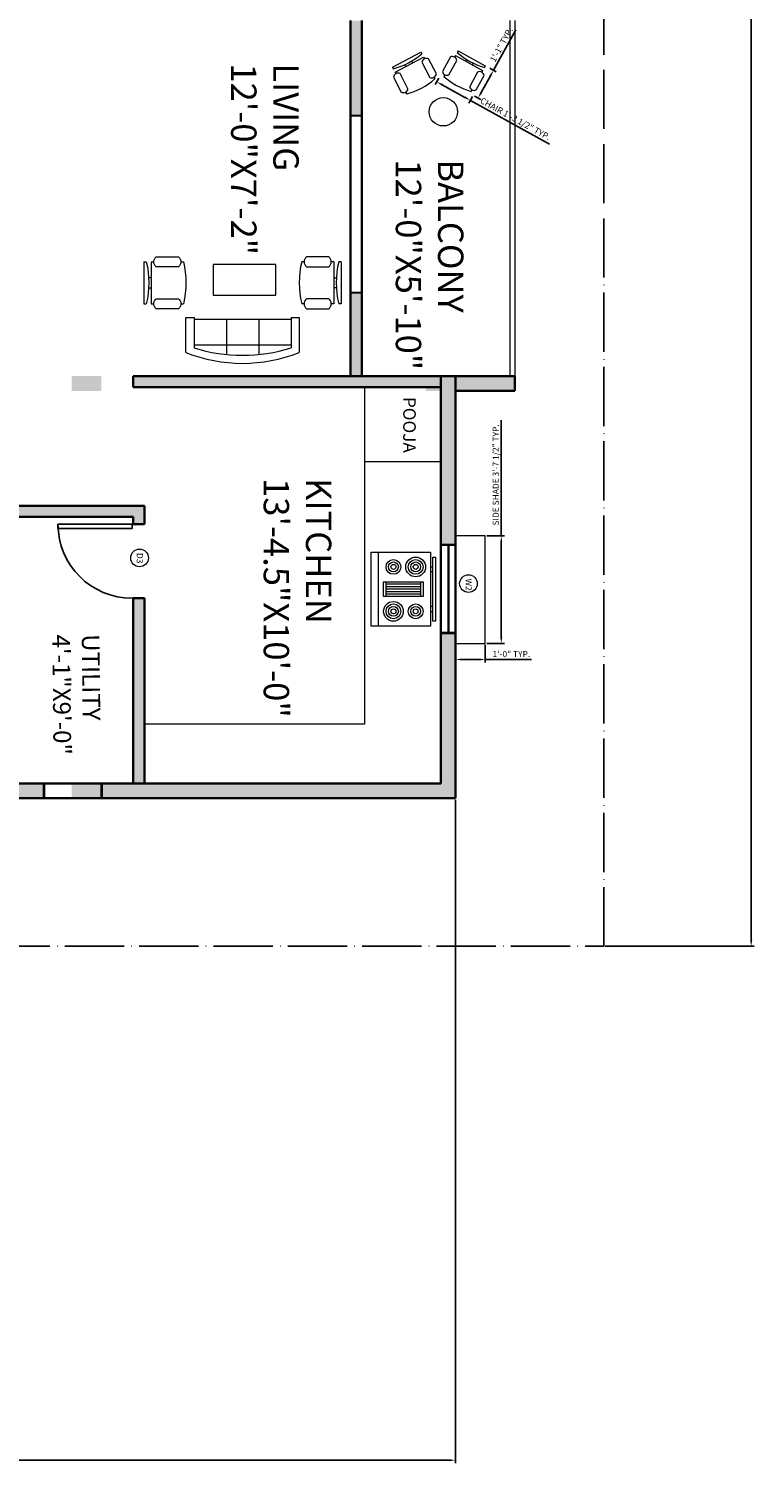
# Model space of a CAD drawing. Units: inches. Extents: x 7028582 to 7030319, y 63109697 to 63111305.
# Tile 7 of 18: x 7030003 to 7030297, y 63109697 to 63110278. Entities that reach past the tile are written whole.
import ezdxf

# ---------------------------------------------------------------- set-up
doc = ezdxf.new("R2010")
doc.units = ezdxf.units.IN
doc.linetypes.add('ACAD_ISO04W100', pattern=[30, 24, -3, 0, -3])
for name, color, linetype, lineweight in [('A-AREA-IDEN', 7, 'Continuous', 18), ('A-DOOR-IDEN', 20, 'Continuous', 13), ('A-EQPM', 9, 'Continuous', 18), ('A-FLOR-CASE', 9, 'Continuous', 18), ('A-FLOR-HRAL', 5, 'Continuous', 18), ('A-GLAZ-IDEN', 20, 'Continuous', 13), ('A-WALL-PATT', 8, 'Continuous', 13), ('C-ANNO-DIMS', 7, 'Continuous', 18), ('C-PROP', 1, 'ACAD_ISO04W100', 25), ('doors', 20, 'Continuous', 25), ('furniture', 9, 'Continuous', 18), ('S-COLS-PATT', 220, 'Continuous', 100), ('walls', 6, 'Continuous', 35), ('WINDOW SHADOW', 9, 'Continuous', 13), ('windows', 5, 'Continuous', 18)]:
    doc.layers.add(name, color=color, linetype=linetype, lineweight=lineweight)
doc.styles.get("Standard").update_dxf_attribs({"font": 'arial.ttf'})
doc.dimstyles.new('ISO-25', dxfattribs={"dimtxt": 2.5, "dimasz": 2.5, "dimexe": 1.25, "dimexo": 0.625, "dimtad": 1, "dimlunit": 4, "dimtxsty": 'Standard', "dimcen": 2.5, "dimadec": 0, "dimazin": 0, "dimtfac": 1, "dimtmove": 0, "dimatfit": 3, "dimfxl": 1, "dimarcsym": 0})

# ---------------------------------------------------------------- blocks, each defined once
blk = doc.blocks.new('*U2')
for p, q in [((0, 0), (0, -5)), ((30, 0), (30, -5))]:
    blk.add_line(p, q)
blk.add_lwpolyline([(0, 0), (0, 30), (1.75, 30), (1.75, 0)], close=True)
blk.add_arc((0, 0), 30, 0, 90)
blk = doc.blocks.new('Range-Oven - 30 in top')
for p, q in [((0, -3), (30, -3)), ((12, -6), (18, -6)), ((13, -20), (13, -6)), ((14, -6), (14, -20)), ((15, -20), (15, -6)), ((16, -6), (16, -20)), ((17, -20), (17, -6)), ((18, -20), (12, -20)), ((6, -24), (6, -25)), ((8, -25), (8, -24)), ((22, -25), (22, -24)), ((24, -24), (24, -25))]:
    blk.add_line(p, q)
for points in [[(0, -24), (0, 0), (30, 0), (30, -24)], [(12, -21), (12, -5), (18, -5), (18, -21)], [(2, -26), (2, -25), (28, -25), (28, -26)]]:
    blk.add_lwpolyline(points, close=True)
for centre, radius in [((6, -9), 4), ((6, -9), 3), ((6, -9), 2), ((6, -9), 1), ((24, -9), 3), ((24, -9), 2), ((24, -9), 1), ((6, -18), 3), ((6, -18), 2), ((6, -18), 1), ((24, -18), 4), ((24, -18), 3), ((24, -18), 2), ((24, -18), 1)]:
    blk.add_circle(centre, radius)
blk = doc.blocks.new('Chair - Desk')
for p, q in [((-8.5, 0), (-8.5, -1)), ((-8.5, 0), (8.5, 0)), ((8.5, 0), (8.5, -1)), ((-10.5, -5), (-10.5, -14)), ((-8.5, -3), (-8.5, -4)), ((-8.5, -3), (8.5, -3)), ((-6.5, -14), (-6.5, -5)), ((-2, -3), (-2, -1.9355)), ((2, -1.9576), (2, -3)), ((6.5, -5), (6.5, -14)), ((8.5, -3), (8.5, -4)), ((10.5, -14), (10.5, -5)), ((-8.5, -15), (-8.5, -16)), ((8.5, -15), (8.5, -16))]:
    blk.add_line(p, q)
for centre, radius, start, end in [((-8.5, -6.5), 2.5, 36.8699, 143.1301), ((0, 34.625), 36.625, 256.5803, 283.4197), ((8.5, -6.5), 2.5, 36.8699, 143.1301), ((-8.5, -12.5), 2.5, 216.8699, 323.1301), ((0, 19.625), 36.625, 256.5803, 283.4197), ((8.5, -12.5), 2.5, 216.8699, 323.1301)]:
    blk.add_arc(centre, radius, start, end)
blk = doc.blocks.new('Sofa - Roundback 7 ft.')
for p, q in [((-12.00002, -32.4421), (-12.00003, -6.5971)), ((11.99997, -32.4421), (11.99998, -6.5971)), ((-36.000027, -34), (-36.000027, -11.4696)), ((-35.999844, -13.3819), (35.9998, -13.3819)), ((35.99998, -34), (35.99998, -11.4696)), ((-36.000027, -32.4421), (35.99998, -32.4421))]:
    blk.add_line(p, q)
for points in [[(-36.000027, -34), (-42.000027, -34), (-42.000027, -8)], [(41.99998, -8), (41.99998, -34), (35.99998, -34)]]:
    blk.add_lwpolyline(points)
for centre, radius, start, end in [((0, -114.25), 114.25, 68.43141, 111.5686), ((-0.00001, -127.1968), 121.1968, 72.72033, 107.2797)]:
    blk.add_arc(centre, radius, start, end)
blk = doc.blocks.new('*D10')
at = {"layer": 'C-ANNO-DIMS', "color": 0, "lineweight": -2, "transparency": 16777216}
for p, q in [((7030236.33, 63111093.06), (7030296.71, 63111093.06)), ((7030295.46, 63111090.56), (7030295.46, 63109909.06)), ((7030236.33, 63109906.56), (7030296.71, 63109906.56))]:
    blk.add_line(p, q, dxfattribs=at)
at = {"layer": 'C-ANNO-DIMS', "color": 0, "lineweight": 100, "transparency": 16777216}
for points in [[(7030295.04, 63111090.56), (7030295.88, 63111090.56), (7030295.46, 63111093.06)], [(7030295.04, 63109909.06), (7030295.88, 63109909.06), (7030295.46, 63109906.56)]]:
    blk.add_solid(points, dxfattribs=at)
at = {"layer": 'Defpoints', "color": 0, "lineweight": 100, "transparency": 16777216}
for p in [(7030235.71, 63111093.06), (7030235.71, 63109906.56), (7030295.46, 63109906.56)]:
    blk.add_point(p, dxfattribs=at)
at = {"layer": 'C-ANNO-DIMS', "color": 0, "transparency": 16777216, "insert": (7030280.69, 63110499.81), "char_height": 12, "attachment_point": 5, "rotation": 90}
blk.add_mtext('98\'-10{\\H1x;\\S1/2;}"', dxfattribs=at)
blk = doc.blocks.new('WIN-SASH-36')
for p, q in [((0, 36.05), (0, 0)), ((6, 35.55), (0, 35.55)), ((2.8, 35.55), (2.8, 0.5)), ((3.2, 35.55), (3.2, 0.5)), ((6, 0), (6, 36.05)), ((0, 0.5), (6, 0.5))]:
    blk.add_line(p, q)
blk = doc.blocks.new('WIN-SASH-24-FRAME')
for p, q in [((24.05, 6), (0, 6)), ((0.5, 6), (0.5, 0)), ((23.55, 0), (23.55, 6)), ((0, 0), (24.05, 0))]:
    blk.add_line(p, q)
blk = doc.blocks.new('WIN-SASH-BALCONY')
for p, q in [((0.13, 72.09), (0.13, 36.05)), ((4.63, 71.71), (0.13, 71.71)), ((4.63, 36.05), (4.63, 72.09)), ((0, 0.02), (0.13, 36.05)), ((0.13, 35.68), (0.13, 35.68)), ((4.63, 36.04), (4.5, 0)), ((4.5, 0.37), (0, 0.39))]:
    blk.add_line(p, q)
blk = doc.blocks.new('WINDOW-SHADE-SIDE-44')
for p, q in [((12, 43.55), (0, 43.55)), ((12, 0), (12, 43.55)), ((0, 0), (12, 0))]:
    blk.add_line(p, q)
blk = doc.blocks.new('KITCHEN-COUNTER')
for p, q in [((89.09, 136.54), (89.09, 16.65)), ((120, 106.35), (89.09, 106.35)), ((89.09, 16.65), (89.09, 0)), ((89.09, 0), (0, 0))]:
    blk.add_line(p, q)
blk = doc.blocks.new('BALCONY-GUARD-12FT')
for p, q in [((0, 144), (0, 0)), ((2, 144), (2, 0))]:
    blk.add_line(p, q)
blk = doc.blocks.new('TABLE-COFFEE-RECT')
blk.add_lwpolyline([(25.34, 12.34), (0, 12.34), (0, 0), (25.34, 0)], close=True)
blk = doc.blocks.new('TAG-D3-MT-R')
blk.add_circle((3.58, 3.58), 3.58)
at = {"insert": (4.93, 5.6), "char_height": 2.5, "attachment_point": 1, "rotation": 270}
blk.add_mtext_dynamic_manual_height_columns('D3', width=2.5021, gutter_width=12.5, heights=[0], dxfattribs=at)
blk = doc.blocks.new('TAG-W2-MT-R')
blk.add_circle((3.58, 3.58), 3.58)
at = {"insert": (4.93, 5.6), "char_height": 2.5, "attachment_point": 1, "rotation": 270}
blk.add_mtext_dynamic_manual_height_columns('W2', width=2.5021, gutter_width=12.5, heights=[0], dxfattribs=at)
blk = doc.blocks.new('TABLE-BALCONY-ROUND')
blk.add_circle((5.75, 5.75), 5.75)
blk = doc.blocks.new('*D51')
at = {"layer": 'C-ANNO-DIMS', "color": 0, "lineweight": -2, "transparency": 16777216}
for p, q in [((7030168.91, 63110258.28), (7030167.48, 63110255.69)), ((7030170.28, 63110255.57), (7030179.52, 63110250.47)), ((7030182.54, 63110250.76), (7030181.11, 63110248.17)), ((7030181.71, 63110249.26), (7030213.77, 63110231.56))]:
    blk.add_line(p, q, dxfattribs=at)
at = {"layer": 'C-ANNO-DIMS', "color": 0, "lineweight": 100, "transparency": 16777216}
for points in [[(7030170.48, 63110255.94), (7030170.08, 63110255.21), (7030168.09, 63110256.78)], [(7030179.72, 63110250.84), (7030179.32, 63110250.11), (7030181.71, 63110249.26)]]:
    blk.add_solid(points, dxfattribs=at)
at = {"layer": 'Defpoints', "color": 0, "lineweight": 100, "transparency": 16777216}
for p in [(7030169.22, 63110258.83), (7030181.71, 63110249.26), (7030182.84, 63110251.31)]:
    blk.add_point(p, dxfattribs=at)
at = {"layer": 'C-ANNO-DIMS', "color": 0, "transparency": 16777216, "insert": (7030199.76, 63110241.49), "char_height": 2.5, "attachment_point": 5, "rotation": 331.10029}
blk.add_mtext('CHAIR 1\'-3 1/2" TYP.', dxfattribs=at)
blk = doc.blocks.new('*D52')
at = {"layer": 'C-ANNO-DIMS', "color": 0, "lineweight": -2, "transparency": 16777216}
for p, q in [((7030191.09, 63110261.42), (7030200.15, 63110277.84)), ((7030186.09, 63110252.37), (7030189.88, 63110259.23)), ((7030189.59, 63110262.25), (7030192.18, 63110260.82)), ((7030183.39, 63110251), (7030185.98, 63110249.57))]:
    blk.add_line(p, q, dxfattribs=at)
at = {"layer": 'C-ANNO-DIMS', "color": 0, "lineweight": 100, "transparency": 16777216}
for points in [[(7030189.52, 63110259.43), (7030190.24, 63110259.03), (7030191.09, 63110261.42)], [(7030185.72, 63110252.57), (7030186.45, 63110252.17), (7030184.88, 63110250.18)]]:
    blk.add_solid(points, dxfattribs=at)
at = {"layer": 'Defpoints', "color": 0, "lineweight": 100, "transparency": 16777216}
for p in [(7030189.04, 63110262.55), (7030191.09, 63110261.42), (7030182.84, 63110251.31)]:
    blk.add_point(p, dxfattribs=at)
at = {"layer": 'C-ANNO-DIMS', "color": 0, "transparency": 16777216, "insert": (7030194.58, 63110271.63), "char_height": 2.5, "attachment_point": 5, "rotation": 61.10029}
blk.add_mtext('1\'-1" TYP.', dxfattribs=at)
blk = doc.blocks.new('*D71')
at = {"layer": 'C-ANNO-DIMS', "color": 0, "lineweight": -2, "transparency": 16777216}
for p, q in [((7030194.24, 63110072.83), (7030194.24, 63110119.76)), ((7030188.33, 63110072.83), (7030195.49, 63110072.83)), ((7030194.24, 63110031.78), (7030194.24, 63110070.33)), ((7030188.33, 63110029.28), (7030195.49, 63110029.28))]:
    blk.add_line(p, q, dxfattribs=at)
at = {"layer": 'C-ANNO-DIMS', "color": 0, "lineweight": 100, "transparency": 16777216}
for points in [[(7030193.82, 63110070.33), (7030194.65, 63110070.33), (7030194.24, 63110072.83)], [(7030193.82, 63110031.78), (7030194.65, 63110031.78), (7030194.24, 63110029.28)]]:
    blk.add_solid(points, dxfattribs=at)
at = {"layer": 'Defpoints', "color": 0, "lineweight": 100, "transparency": 16777216}
for p in [(7030187.71, 63110072.83), (7030194.24, 63110072.83), (7030187.71, 63110029.28)]:
    blk.add_point(p, dxfattribs=at)
at = {"layer": 'C-ANNO-DIMS', "color": 0, "transparency": 16777216, "insert": (7030192.32, 63110097.54), "char_height": 2.5, "attachment_point": 5, "rotation": 90}
blk.add_mtext('SIDE SHADE 3\'-7 1/2" TYP.', dxfattribs=at)
blk = doc.blocks.new('*D72')
at = {"layer": 'C-ANNO-DIMS', "color": 0, "lineweight": -2, "transparency": 16777216}
for p, q in [((7030175.71, 63110028.66), (7030175.71, 63110021.5)), ((7030187.71, 63110028.66), (7030187.71, 63110021.5)), ((7030178.21, 63110022.75), (7030185.21, 63110022.75)), ((7030187.71, 63110022.75), (7030206.46, 63110022.75))]:
    blk.add_line(p, q, dxfattribs=at)
at = {"layer": 'C-ANNO-DIMS', "color": 0, "lineweight": 100, "transparency": 16777216}
for points in [[(7030178.21, 63110023.16), (7030178.21, 63110022.33), (7030175.71, 63110022.75)], [(7030185.21, 63110023.16), (7030185.21, 63110022.33), (7030187.71, 63110022.75)]]:
    blk.add_solid(points, dxfattribs=at)
at = {"layer": 'Defpoints', "color": 0, "lineweight": 100, "transparency": 16777216}
for p in [(7030175.71, 63110029.28), (7030187.71, 63110029.28), (7030187.71, 63110022.75)]:
    blk.add_point(p, dxfattribs=at)
at = {"layer": 'C-ANNO-DIMS', "color": 0, "transparency": 16777216, "insert": (7030198.33, 63110024.65), "char_height": 2.5, "attachment_point": 5}
blk.add_mtext('1\'-0" TYP.', dxfattribs=at)
blk = doc.blocks.new('*D99')
at = {"layer": 'C-ANNO-DIMS', "color": 0, "lineweight": -2, "transparency": 16777216}
for p, q in [((7029234.71, 63109965.93), (7029234.71, 63109697.14)), ((7030175.71, 63109965.93), (7030175.71, 63109697.14)), ((7029237.21, 63109698.39), (7030173.21, 63109698.39))]:
    blk.add_line(p, q, dxfattribs=at)
at = {"layer": 'C-ANNO-DIMS', "color": 0, "lineweight": 100, "transparency": 16777216}
for points in [[(7029237.21, 63109698.8), (7029237.21, 63109697.97), (7029234.71, 63109698.39)], [(7030173.21, 63109698.8), (7030173.21, 63109697.97), (7030175.71, 63109698.39)]]:
    blk.add_solid(points, dxfattribs=at)
at = {"layer": 'Defpoints', "color": 0, "lineweight": 100, "transparency": 16777216}
for p in [(7029234.71, 63109966.56), (7030175.71, 63109966.56), (7030175.71, 63109698.39)]:
    blk.add_point(p, dxfattribs=at)
at = {"layer": 'C-ANNO-DIMS', "color": 0, "transparency": 16777216, "insert": (7029705.21, 63109700.29), "char_height": 2.5, "attachment_point": 5}
blk.add_mtext('78\'-5"', dxfattribs=at)

msp = doc.modelspace()

# ---------------------------------------------------------------- hatches: boundary and pattern name
at = {"layer": 'A-WALL-PATT'}
h = msp.add_hatch(color=256, dxfattribs=at)
h.dxf.hatch_style = 1
h.paths.add_polyline_path([(7030137.705, 63110281.557), (7030133.205, 63110281.557), (7030133.205, 63110243.163), (7030137.705, 63110243.163)])
h = msp.add_hatch(color=256, dxfattribs=at)
h.dxf.hatch_style = 1
h.paths.add_polyline_path([(7030137.705, 63110171.074), (7030133.205, 63110171.09), (7030133.205, 63110137.557), (7030137.705, 63110137.557)])
h = msp.add_hatch(color=256, dxfattribs=at)
h.dxf.hatch_style = 1
h.paths.add_polyline_path([(7030169.705, 63110137.557), (7030045.205, 63110137.557), (7030045.205, 63110133.057), (7030169.705, 63110133.057)])
h = msp.add_hatch(color=256, dxfattribs=at)
h.dxf.hatch_style = 1
h.paths.add_polyline_path([(7030175.705, 63110137.557), (7030169.705, 63110137.557), (7030169.705, 63110069.386), (7030175.705, 63110069.386)])
h = msp.add_hatch(color=256, dxfattribs=at)
h.dxf.hatch_style = 1
h.paths.add_polyline_path([(7030199.705, 63110137.557), (7030175.705, 63110137.557), (7030175.705, 63110131.557), (7030199.705, 63110131.557)])
h = msp.add_hatch(color=256, dxfattribs=at)
h.dxf.hatch_style = 1
h.paths.add_polyline_path([(7030049.705, 63110085.057), (7029996.205, 63110085.057), (7029996.205, 63110080.557), (7030045.205, 63110080.557), (7030045.205, 63110077.557), (7030049.705, 63110077.557)])
h = msp.add_hatch(color=256, dxfattribs=at)
h.dxf.hatch_style = 1
h.paths.add_polyline_path([(7029996.205, 63110080.557), (7029991.705, 63110080.557), (7029991.705, 63109972.557), (7029973.979, 63109972.557), (7029973.979, 63109966.557), (7030008.697, 63109966.557), (7030008.697, 63109972.557), (7029996.205, 63109972.557)])
h = msp.add_hatch(color=256, dxfattribs=at)
h.dxf.hatch_style = 1
h.paths.add_polyline_path([(7030175.705, 63110033.338), (7030169.705, 63110033.338), (7030169.705, 63109972.557), (7030049.705, 63109972.557), (7030049.705, 63110047.557), (7030045.205, 63110047.557), (7030045.205, 63109972.557), (7030032.745, 63109972.557), (7030032.745, 63109966.557), (7030175.705, 63109966.557)])
at = {"layer": 'S-COLS-PATT'}
h = msp.add_hatch(color=256, dxfattribs=at)
h.dxf.hatch_style = 1
h.paths.add_polyline_path([(7030032.194, 63110137.557), (7030020.279, 63110137.557), (7030020.279, 63110131.557), (7030032.194, 63110131.557)])
h = msp.add_hatch(color=256, dxfattribs=at)
h.dxf.hatch_style = 1
h.paths.add_polyline_path([(7030175.705, 63110137.557), (7030163.791, 63110137.557), (7030163.791, 63110131.557), (7030175.705, 63110131.557)])
h = msp.add_hatch(color=256, dxfattribs=at)
h.dxf.hatch_style = 1
h.paths.add_polyline_path([(7030032.194, 63109972.505), (7030020.279, 63109972.505), (7030020.279, 63109966.505), (7030032.194, 63109966.505)])
h = msp.add_hatch(color=256, dxfattribs=at)
h.dxf.hatch_style = 1
h.paths.add_polyline_path([(7030175.705, 63109972.505), (7030163.791, 63109972.505), (7030163.791, 63109966.505), (7030175.705, 63109966.505)])

# ---------------------------------------------------------------- linework, layer by layer
at = {"layer": 'C-PROP'}
for p, q in [((7030235.705, 63109906.557), (7030235.705, 63111093.057)), ((7029174.705, 63109906.557), (7030235.705, 63109906.557))]:
    msp.add_line(p, q, dxfattribs=at)
at = {"layer": 'walls'}
for p, q in [((7030133.205, 63110281.557), (7030133.205, 63110137.557)), ((7030137.705, 63110281.557), (7030137.705, 63110137.557)), ((7030045.205, 63110133.057), (7030045.205, 63110137.557)), ((7030175.705, 63110137.557), (7030045.205, 63110137.557)), ((7030169.705, 63109972.557), (7030169.705, 63110137.557)), ((7030169.705, 63109972.557), (7030169.705, 63110137.557)), ((7030175.705, 63109966.557), (7030175.705, 63110137.557)), ((7030175.705, 63109966.557), (7030175.705, 63110137.557)), ((7030199.705, 63110137.557), (7030175.705, 63110137.557)), ((7030199.705, 63110131.557), (7030199.705, 63110137.557)), ((7030169.705, 63110133.057), (7030045.205, 63110133.057)), ((7030175.705, 63110131.557), (7030199.705, 63110131.557)), ((7030049.705, 63110085.057), (7029964.705, 63110085.057)), ((7030049.705, 63110077.557), (7030049.705, 63110085.057)), ((7030045.205, 63110080.557), (7029964.705, 63110080.557)), ((7030045.205, 63110077.557), (7030045.205, 63110080.557)), ((7030045.205, 63110080.557), (7030045.205, 63110077.557)), ((7030045.205, 63110077.557), (7030049.705, 63110077.557)), ((7030045.205, 63109972.557), (7030045.205, 63110047.557)), ((7030049.705, 63110047.557), (7030045.205, 63110047.557)), ((7030049.705, 63109972.557), (7030049.705, 63110047.557)), ((7029240.705, 63109972.557), (7030169.705, 63109972.557)), ((7030169.705, 63109972.557), (7029240.705, 63109972.557)), ((7030045.205, 63109972.557), (7029996.205, 63109972.557)), ((7030169.705, 63109972.557), (7030049.705, 63109972.557)), ((7029234.705, 63109966.557), (7030175.705, 63109966.557)), ((7030175.705, 63109966.557), (7029234.705, 63109966.557)), ((7030175.705, 63109966.557), (7029748.205, 63109966.557))]:
    msp.add_line(p, q, dxfattribs=at)
at = {"layer": 'windows'}
for p, q in [((7030137.705, 63110243.163), (7030133.205, 63110243.163)), ((7030137.577, 63110171.074), (7030133.077, 63110171.09)), ((7030175.898, 63110069.386), (7030169.898, 63110069.386)), ((7030169.898, 63110033.338), (7030175.898, 63110033.338)), ((7030008.697, 63109972.557), (7030008.697, 63109966.557)), ((7030032.745, 63109966.557), (7030032.745, 63109972.557))]:
    msp.add_line(p, q, dxfattribs=at)

# ---------------------------------------------------------------- block references
at = {"layer": 'A-DOOR-IDEN'}
msp.add_blockref('TAG-D3-MT-R', (7030044.153, 63110060.309), dxfattribs=at)
at = {"layer": 'A-EQPM', "rotation": 90}
msp.add_blockref('Range-Oven - 30 in top', (7030141.566, 63110036.257), dxfattribs=at)
at = {"layer": 'A-FLOR-CASE'}
msp.add_blockref('KITCHEN-COUNTER', (7030049.705, 63109996.518), dxfattribs=at)
at = {"layer": 'A-FLOR-HRAL'}
msp.add_blockref('BALCONY-GUARD-12FT', (7030197.705, 63110137.557), dxfattribs=at)
at = {"layer": 'A-GLAZ-IDEN'}
msp.add_blockref('TAG-W2-MT-R', (7030177.373, 63110049.907), dxfattribs=at)
at = {"layer": 'doors', "xscale": -1, "rotation": 90}
msp.add_blockref('*U2', (7030044.705, 63110077.557), dxfattribs=at)
at = {"layer": 'furniture'}
for name, p, xscale, yscale, zscale, rotation in [('Chair - Desk', (7030155.914, 63110265.758), 0.7643373636972337, 0.7643373636972337, 0.7643373636972337, 27.52919134002635), ('Chair - Desk', (7030182.234, 63110266.309), 0.740937522274531, 0.740937522274531, 0.740937522274531, 331.1002874626102), ('Sofa - Roundback 7 ft.', (7030089.438, 63110142.72), 0.5455524879488546, 0.5455524879488546, 0.5455524879488546, 180)]:
    msp.add_blockref(name, p, dxfattribs=dict(at, xscale=xscale, yscale=yscale, zscale=zscale, rotation=rotation))
for name, p in [('TABLE-BALCONY-ROUND', (7030165.023, 63110238.874)), ('TABLE-COFFEE-RECT', (7030077.552, 63110170.363))]:
    msp.add_blockref(name, p, dxfattribs=at)
at = {"layer": 'furniture', "xscale": -1, "rotation": 90}
msp.add_blockref('Chair - Desk', (7030049.481, 63110175.367), dxfattribs=at)
at = {"layer": 'furniture', "rotation": 270}
msp.add_blockref('Chair - Desk', (7030129.395, 63110175.367), dxfattribs=at)
at = {"layer": 'WINDOW SHADOW'}
msp.add_blockref('WINDOW-SHADE-SIDE-44', (7030175.705, 63110029.281), dxfattribs=at)
at = {"layer": 'windows'}
for name, p in [('WIN-SASH-BALCONY', (7030133.077, 63110171.074)), ('WIN-SASH-24-FRAME', (7030008.697, 63109966.557))]:
    msp.add_blockref(name, p, dxfattribs=at)
at = {"layer": 'windows', "rotation": 180}
msp.add_blockref('WIN-SASH-36', (7030175.898, 63110069.386), dxfattribs=at)

# ---------------------------------------------------------------- texts
at = {"layer": 'A-AREA-IDEN', "attachment_point": 1}
for s, width, gutter_width, insert, char_height, rotation in [('LIVING\\P12\'-0"X7\'-2"', 82.04322, 51.315, (7030112.192, 63110264.231), 10.26307, 270), ('BALCONY\\P12\'-0"X5\'-10"', 82.04322, 51.315, (7030178.895, 63110225.354), 10.26307, 270), ('POOJA', 15.69653, 25.463, (7030159.602, 63110129.117), 5.0926, 270), ('KITCHEN\\P13\'-4.5"X10\'-0"', 82.04322, 51.315, (7030125.386, 63110096.255), 10.26307, 270), ('UTILITY\\P4\'-1"X9\'-0"', 42.97461, 35.821, (7030031.482, 63110033.048), 7.16426, 270.646399)]:
    msp.add_mtext_dynamic_manual_height_columns(s, width=width, gutter_width=gutter_width, heights=[0], dxfattribs=dict(at, insert=insert, char_height=char_height, rotation=rotation))

# ---------------------------------------------------------------- dimensions: what is measured, and where the dimension line sits
at = {"layer": 'C-ANNO-DIMS'}
dim = msp.add_linear_dim(base=(7030295.462, 63109906.557), p1=(7030235.705, 63111093.057), p2=(7030235.705, 63109906.557), angle=90, dimstyle='ISO-25', override={"dimtxt": 12, "dimclrd": 0, "dimclre": 0, "dimclrt": 0}, dxfattribs=at)
dim.commit()
dim.dimension.update_dxf_attribs({"geometry": '*D10', "text_midpoint": (7030280.685, 63110499.807)})
for base, p1, p2, angle, text, picture, middle in [((7030191.088, 63110261.421), (7030182.838, 63110251.306), (7030189.045, 63110262.549), 61.100287, '<> TYP.', '*D52', (7030194.577, 63110271.634)), ((7030181.71, 63110249.262), (7030169.216, 63110258.825), (7030182.838, 63110251.306), 331.100287, 'CHAIR <> TYP.', '*D51', (7030199.762, 63110241.489)), ((7030194.238, 63110072.829), (7030187.705, 63110029.281), (7030187.705, 63110072.829), 90, 'SIDE SHADE <> TYP.', '*D71', (7030192.319, 63110097.542))]:
    dim = msp.add_linear_dim(base=base, p1=p1, p2=p2, angle=angle, text=text, dimstyle='ISO-25', override={"dimdec": 1, "dimlfac": 1, "dimrnd": 0, "dimzin": 1, "dimdsep": 46, "dimlunit": 4, "dimfrac": 2}, dxfattribs=at)
    dim.commit()
    dim.dimension.update_dxf_attribs({"geometry": picture, "text_midpoint": middle})
dim = msp.add_linear_dim(base=(7030187.705, 63110022.748), p1=(7030175.705, 63110029.281), p2=(7030187.705, 63110029.281), text='<> TYP.', dimstyle='ISO-25', override={"dimdec": 1, "dimlfac": 1, "dimrnd": 0, "dimzin": 1, "dimdsep": 46, "dimlunit": 4, "dimfrac": 2}, dxfattribs=at)
dim.commit()
dim.dimension.update_dxf_attribs({"geometry": '*D72', "text_midpoint": (7030198.332, 63110024.65)})
dim = msp.add_linear_dim(base=(7030175.705, 63109698.385), p1=(7029234.705, 63109966.557), p2=(7030175.705, 63109966.557), dimstyle='ISO-25', override={"dimdec": 1, "dimlfac": 1, "dimrnd": 0, "dimzin": 1, "dimdsep": 46, "dimlunit": 4, "dimfrac": 2}, dxfattribs=at)
dim.commit()
dim.dimension.update_dxf_attribs({"geometry": '*D99', "text_midpoint": (7029705.205, 63109700.287)})

doc.saveas('drawing.dxf')
